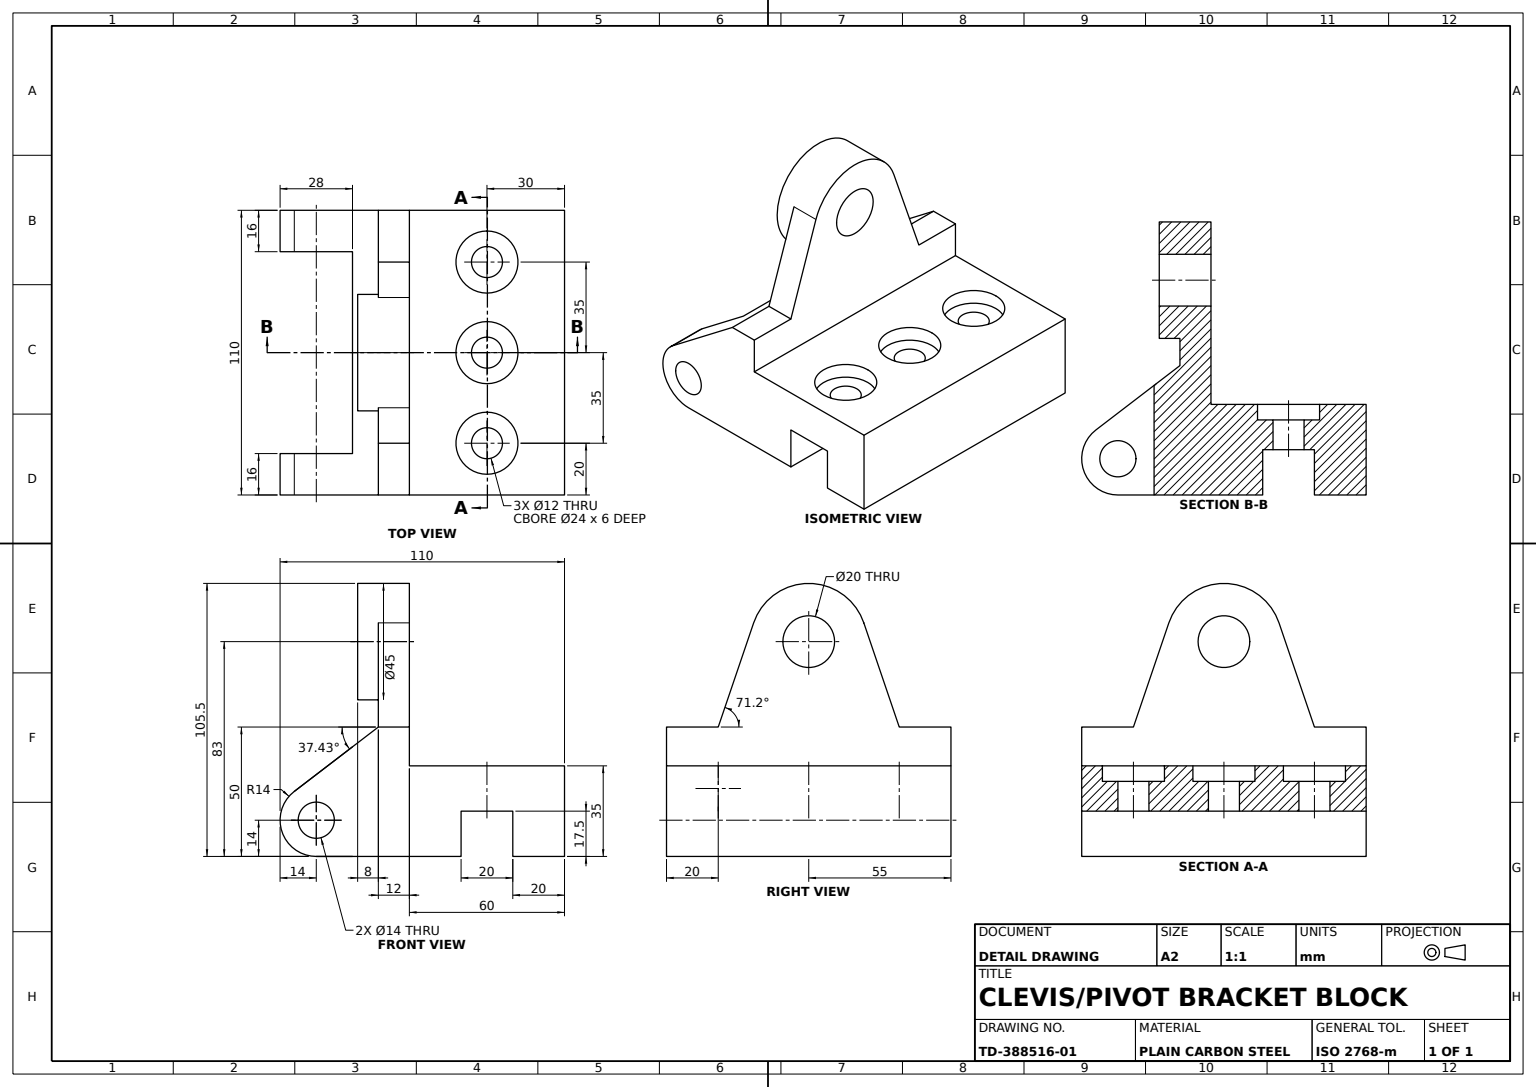
from build123d import *

# Parameters (mm, degrees)
BASE_PROFILE_SKETCH_R                = 7
BASE_BLOCK_DEPTH                     = 55
GUIDE_SLOT_SKETCH_W                  = 28
GUIDE_SLOT_SKETCH_H                  = 78
GUIDE_SLOT_16X16_DEPTH               = 110
PIVOT_LUG_SKETCH_R                   = 10
PIVOT_LUG_DEPTH                      = 12
LUG_SUPPORT_SKETCH_R                 = 22.5
LUG_SUPPORT_SKETCH_R_2               = 10
LUG_SUPPORT_BOSS_DEPTH               = 8
COUNTERBORED_HOLES_3X_12_D           = 12
COUNTERBORED_HOLES_3X_12_DEPTH       = 99.819837708
COUNTERBORED_HOLES_3X_12_CBORE_D     = 24
COUNTERBORED_HOLES_3X_12_CBORE_DEPTH = 6


with BuildPart() as part:
    # Base Profile Sketch → Base Block (new, symmetric)
    with BuildSketch(Plane.XY):
        with BuildLine():
            Line((0, -14), (56, -14))
            Line((56, -14), (56, 3.5))
            Line((56, 3.5), (76, 3.5))
            Line((76, 3.5), (76, -14))
            Line((76, -14), (96, -14))
            Line((96, -14), (96, 21))
            Line((96, 21), (36, 21))
            Line((36, 21), (36, 36))
            Line((36, 36), (24, 36))
            Line((24, 36), (-8.50921229, 11.117252638))
            ThreePointArc((-8.50921229, 11.117252638), (-13.259742398, -4.492129955), (0, -14))
        make_face()
        Circle(BASE_PROFILE_SKETCH_R, mode=Mode.SUBTRACT)
    extrude(amount=BASE_BLOCK_DEPTH, both=True)

    # Guide Slot Sketch → Guide Slot 16x16 (cut)
    with BuildSketch(Plane.XZ.offset(14)):
        Rectangle(GUIDE_SLOT_SKETCH_W, GUIDE_SLOT_SKETCH_H)
    extrude(amount=-GUIDE_SLOT_16X16_DEPTH, mode=Mode.SUBTRACT)

    # Pivot Lug Sketch → Pivot Lug (add)
    with BuildSketch(Plane(origin=(36, 0, 0), x_dir=(0, 0, -1), z_dir=(1, 0, 0))):
        with BuildLine():
            Line((35, 36), (21.299956881, 76.249954267))
            ThreePointArc((21.299956881, 76.249954267), (0, 91.5), (-21.299956881, 76.249954267))
            Line((-21.299956881, 76.249954267), (-35, 36))
            Line((-35, 36), (35, 36))
        make_face()
        with Locations((0, 69)):
            Circle(PIVOT_LUG_SKETCH_R, mode=Mode.SUBTRACT)
    extrude(amount=-PIVOT_LUG_DEPTH)

    # Lug Support Sketch → Lug Support Boss (add)
    with BuildSketch(Plane.ZY.offset(-24)):
        with Locations(Location((0, 69, 0), (0, 0, 161.202754194))):
            Circle(LUG_SUPPORT_SKETCH_R)
        with Locations(Location((0, 69, 0), (0, 0, 180))):
            Circle(LUG_SUPPORT_SKETCH_R_2, mode=Mode.SUBTRACT)
    extrude(amount=LUG_SUPPORT_BOSS_DEPTH)

    # Counterbored Holes 3xØ12
    with Locations(Plane(origin=(66, 21, 35), x_dir=(1, 0, 0), z_dir=(0, 1, 0))):
        with Locations((0, 0), (0, 35), (0, 70)):
            CounterBoreHole(COUNTERBORED_HOLES_3X_12_D / 2, COUNTERBORED_HOLES_3X_12_CBORE_D / 2, COUNTERBORED_HOLES_3X_12_CBORE_DEPTH, depth=COUNTERBORED_HOLES_3X_12_DEPTH)


solid = part.part
